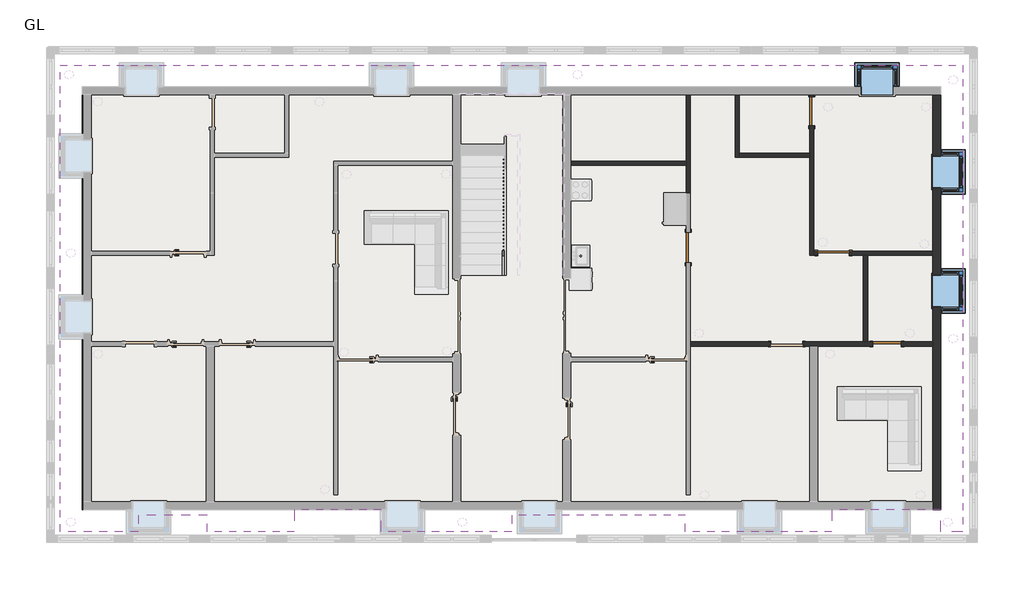
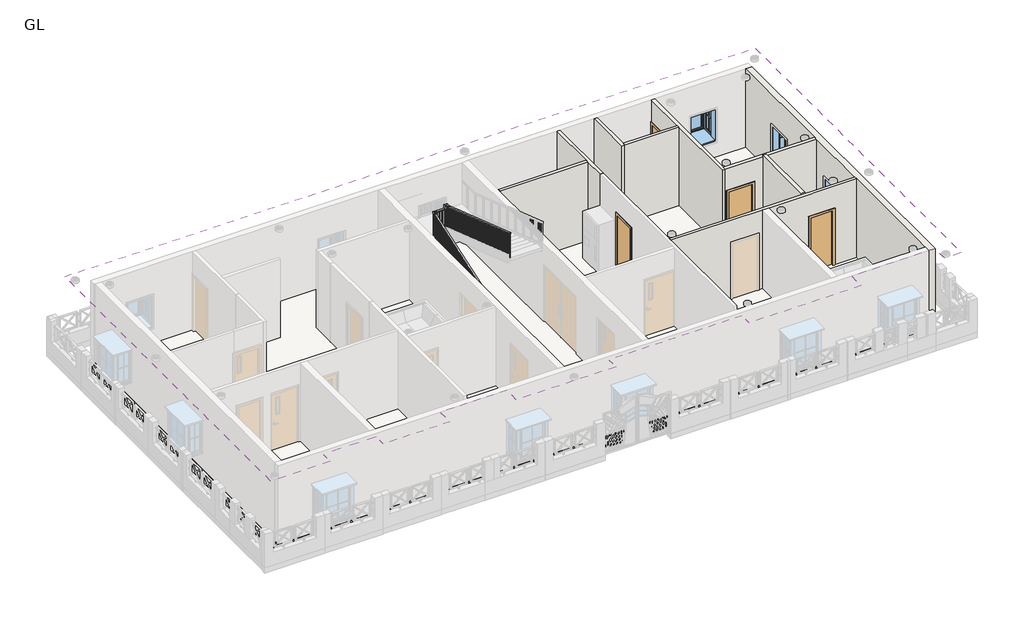
# One storey, part 2 of 5: 10 walls, 4 doors, 3 windows, 1 covering, 1 railing, 1 slab.
"""IFC4 building model written with IfcOpenShell, lengths in millimetres."""

from ifc_helpers import new_model, si_unit, frame, origin, origin_with_axes, place, context, project, spatial, polyline, outline, extrude, faceted_brep, transform, mapped, element, save
from components import door_700d3439, door_8cb1b8a7, door_38851409, door_d141acb4, window_bay_casement_box_90_degree_angle_center_fixed_4_x3_2dea7aab

model = new_model("IFC4")

# Units and contexts
model_context = context("Model", 3, world=origin())
ifc_project = project(units=[si_unit("LENGTHUNIT", "METRE", prefix="MILLI")], contexts=[model_context])

# Site, building, storey
site = spatial("IfcSite", under=ifc_project)
building = spatial("IfcBuilding", under=site)
storey = spatial("IfcBuildingStorey", under=building, Name="GL", Elevation=0.0)

# Covering
placement = place(None, origin())
element("IfcCovering", 1, ObjectType="2' x 4' ACT System", at=placement, inside=storey, context=model_context, shape_type="SweptSolid", body=[
    extrude(outline(polyline([(12235.5012075, 8470.0067329), (12235.5012075, -4623.6932193), (11625.9012075, -4623.6932193), (11625.9012075, -4014.0932193), (8564.9472043, -4014.0932193), (8564.9472043, -4623.6932193), (4450.1472043, -4623.6932193), (4450.1472043, -4172.8432432), (-426.6527957, -4172.8432432), (-426.6527957, -4623.6932193), (-4084.2527957, -4623.6932193), (-4084.2527957, -4014.0932193), (-6522.6527957, -4014.0932193), (-6522.6527957, -4623.6932193), (-8961.0527957, -4623.6932193), (-8961.0527957, -4172.8432432), (-10904.4067989, -4172.8432432), (-10904.4067989, -4623.6932193), (-13088.8067989, -4623.6932193), (-13088.8067989, 8470.0067329), (12235.5012075, 8470.0067329)])), frame((0.0, 0.0, 3048.0), z_axis=(0.0, 0.0, 1.0), x_axis=(1.0, 0.0, 0.0)), (0.0, 0.0, 1.0), 57.15),
])

# Doors
door_shape = door_700d3439(model_context)
element("IfcDoor", 2, ObjectType="Single-Flush : 2'10\" x 7'", at=placement, inside=storey, context=model_context, shape_type="MappedRepresentation", body=[
    mapped(door_shape, transform((4532.9512082, 3351.906733, 0.0), x_axis=(0.0, -1.0, 0.0), y_axis=(1.0, 0.0, 0.0), z_axis=(0.0, 0.0, 1.0))),
])
door_2_shape = door_8cb1b8a7(model_context)
element("IfcDoor", 3, ObjectType="Single-Flush : 2'11\"x 7'", at=placement, inside=storey, context=model_context, shape_type="MappedRepresentation", body=[
    mapped(door_2_shape, transform((8609.6512079, 3193.1567332, 0.0), x_axis=(-1.0, 0.0, 0.0), y_axis=(0.0, -1.0, 0.0), z_axis=(0.0, 0.0, 1.0))),
])
door_3_shape = door_38851409(model_context)
element("IfcDoor", 4, ObjectType="Single-Flush : 2'8\"x 7'", at=placement, inside=storey, context=model_context, shape_type="MappedRepresentation", body=[
    mapped(door_3_shape, transform((10111.5098918, 640.4567334, 0.0), x_axis=(-1.0, 0.0, 0.0), y_axis=(0.0, -1.0, 0.0), z_axis=(0.0, 0.0, 1.0))),
])
door_4_shape = door_d141acb4(model_context)
element("IfcDoor", 5, ObjectType="Single-Flush : 2'8\"x 7'", at=placement, inside=storey, context=model_context, shape_type="MappedRepresentation", body=[
    mapped(door_4_shape, transform((8000.0512079, 7167.840939, 0.0), x_axis=(0.0, 1.0, 0.0), y_axis=(-1.0, 0.0, 0.0), z_axis=(0.0, 0.0, 1.0))),
])

# Railing
element("IfcRailing", 6, ObjectType="Handrail - Rectangular", at=placement, inside=storey, context=model_context, shape_type="SolidModel", body=[
    faceted_brep([(-680.3987998, 2564.5067329, 1017.8142857), (-680.3987998, 2564.5067329, 964.1699957), (-629.5987998, 2564.5067329, 964.1699957), (-629.5987998, 2564.5067329, 1017.8142857), (-680.3987998, 6450.7067329, 2336.3464286), (-680.3987998, 6501.5067329, 2299.9378529), (-629.5987998, 6501.5067329, 2299.9378529), (-629.5987998, 6450.7067329, 2336.3464286), (-553.3987998, 6577.7067329, 2311.4), (-553.3987998, 6577.7067329, 2362.2), (-273.9987915, 6577.7067329, 2362.2), (-223.1987915, 6577.7067329, 2311.4), (-553.3987998, 6526.9067329, 2311.4), (-223.1987915, 6526.9067329, 2311.4), (-553.3987998, 6526.9067329, 2362.2), (-273.9987915, 6526.9067329, 2362.2), (-146.9987915, 2564.5067329, 3810.0), (-197.7987915, 2564.5067329, 3810.0), (-197.7987915, 2564.5067329, 3756.35571), (-146.9987915, 2564.5067329, 3756.35571), (-146.9987915, 6442.3235624, 2440.6678571), (-146.9987915, 6450.7067329, 2491.4678571), (-197.7987915, 6442.3235624, 2440.6678571), (-197.7987915, 6450.7067329, 2491.4678571), (-680.3987998, 6450.7067329, 2362.2), (-680.3987998, 6501.5067329, 2311.4), (-629.5987998, 6501.5067329, 2311.4), (-629.5987998, 6450.7067329, 2362.2), (-680.3987998, 6577.7067329, 2362.2), (-680.3987998, 6577.7067329, 2311.4), (-629.5987998, 6526.9067329, 2311.4), (-629.5987998, 6526.9067329, 2362.2), (-273.9987915, 6577.7067329, 2491.4678571), (-223.1987915, 6577.7067329, 2440.6678571), (-223.1987915, 6526.9067329, 2440.6678571), (-273.9987915, 6526.9067329, 2491.4678571), (-146.9987915, 6577.7067329, 2491.4678571), (-146.9987915, 6577.7067329, 2440.6678571), (-197.7987915, 6526.9067329, 2440.6678571), (-197.7987915, 6526.9067329, 2491.4678571)], [[[0, 1, 2, 3]], [[1, 0, 4, 5]], [[2, 1, 5, 6]], [[3, 2, 6, 7]], [[0, 3, 7, 4]], [[8, 9, 10, 11]], [[12, 8, 11, 13]], [[14, 12, 13, 15]], [[9, 14, 15, 10]], [[16, 17, 18, 19]], [[20, 21, 16, 19]], [[22, 20, 19, 18]], [[23, 22, 18, 17]], [[21, 23, 17, 16]], [[5, 4, 24, 25]], [[6, 5, 25, 26]], [[7, 6, 26, 27]], [[4, 7, 27, 24]], [[25, 24, 28, 29]], [[26, 25, 29, 30]], [[27, 26, 30, 31]], [[24, 27, 31, 28]], [[29, 28, 9, 8]], [[30, 29, 8, 12]], [[31, 30, 12, 14]], [[28, 31, 14, 9]], [[11, 10, 32, 33]], [[13, 11, 33, 34]], [[15, 13, 34, 35]], [[10, 15, 35, 32]], [[33, 32, 36, 37]], [[34, 33, 37, 38]], [[35, 34, 38, 39]], [[32, 35, 39, 36]], [[37, 36, 21, 20]], [[38, 37, 20, 22]], [[39, 38, 22, 23]], [[36, 39, 23, 21]]]),
    extrude(outline(polyline([(2580.3817329, 3750.9695493), (2599.4317329, 3744.5061565), (2599.4317329, 2792.1857143), (2580.3817329, 2792.1857143), (2580.3817329, 3750.9695493)])), frame((-181.9237915, 0.0, 0.0), z_axis=(1.0, 0.0, 0.0), x_axis=(0.0, 1.0, 0.0)), (0.0, 0.0, 1.0), 19.05),
    extrude(outline(polyline([(2681.9817329, 3716.4981207), (2701.0317329, 3710.0347279), (2701.0317329, 2792.1857143), (2681.9817329, 2792.1857143), (2681.9817329, 3716.4981207)])), frame((-181.9237915, 0.0, 0.0), z_axis=(1.0, 0.0, 0.0), x_axis=(0.0, 1.0, 0.0)), (0.0, 0.0, 1.0), 19.05),
    extrude(outline(polyline([(2783.5817329, 3682.0266922), (2802.6317329, 3675.5632993), (2802.6317329, 2792.1857143), (2783.5817329, 2792.1857143), (2783.5817329, 3682.0266922)])), frame((-181.9237915, 0.0, 0.0), z_axis=(1.0, 0.0, 0.0), x_axis=(0.0, 1.0, 0.0)), (0.0, 0.0, 1.0), 19.05),
    extrude(outline(polyline([(2885.1817329, 3647.5552636), (2904.2317329, 3641.0918707), (2904.2317329, 2688.7714286), (2885.1817329, 2688.7714286), (2885.1817329, 3647.5552636)])), frame((-181.9237915, 0.0, 0.0), z_axis=(1.0, 0.0, 0.0), x_axis=(0.0, 1.0, 0.0)), (0.0, 0.0, 1.0), 19.05),
    extrude(outline(polyline([(2986.7817329, 3613.083835), (3005.8317329, 3606.6204422), (3005.8317329, 2688.7714286), (2986.7817329, 2688.7714286), (2986.7817329, 3613.083835)])), frame((-181.9237915, 0.0, 0.0), z_axis=(1.0, 0.0, 0.0), x_axis=(0.0, 1.0, 0.0)), (0.0, 0.0, 1.0), 19.05),
    extrude(outline(polyline([(3088.3817329, 3578.6124065), (3107.4317329, 3572.1490136), (3107.4317329, 2688.7714286), (3088.3817329, 2688.7714286), (3088.3817329, 3578.6124065)])), frame((-181.9237915, 0.0, 0.0), z_axis=(1.0, 0.0, 0.0), x_axis=(0.0, 1.0, 0.0)), (0.0, 0.0, 1.0), 19.05),
    extrude(outline(polyline([(3189.9817329, 3544.1409779), (3209.0317329, 3537.677585), (3209.0317329, 2585.3571429), (3189.9817329, 2585.3571429), (3189.9817329, 3544.1409779)])), frame((-181.9237915, 0.0, 0.0), z_axis=(1.0, 0.0, 0.0), x_axis=(0.0, 1.0, 0.0)), (0.0, 0.0, 1.0), 19.05),
    extrude(outline(polyline([(3291.5817329, 3509.6695493), (3310.6317329, 3503.2061565), (3310.6317329, 2585.3571429), (3291.5817329, 2585.3571429), (3291.5817329, 3509.6695493)])), frame((-181.9237915, 0.0, 0.0), z_axis=(1.0, 0.0, 0.0), x_axis=(0.0, 1.0, 0.0)), (0.0, 0.0, 1.0), 19.05),
    extrude(outline(polyline([(3393.1817329, 3475.1981207), (3412.2317329, 3468.7347279), (3412.2317329, 2585.3571429), (3393.1817329, 2585.3571429), (3393.1817329, 3475.1981207)])), frame((-181.9237915, 0.0, 0.0), z_axis=(1.0, 0.0, 0.0), x_axis=(0.0, 1.0, 0.0)), (0.0, 0.0, 1.0), 19.05),
    extrude(outline(polyline([(3494.7817329, 3440.7266922), (3513.8317329, 3434.2632993), (3513.8317329, 2481.9428571), (3494.7817329, 2481.9428571), (3494.7817329, 3440.7266922)])), frame((-181.9237915, 0.0, 0.0), z_axis=(1.0, 0.0, 0.0), x_axis=(0.0, 1.0, 0.0)), (0.0, 0.0, 1.0), 19.05),
    extrude(outline(polyline([(3596.3817329, 3406.2552636), (3615.4317329, 3399.7918707), (3615.4317329, 2481.9428571), (3596.3817329, 2481.9428571), (3596.3817329, 3406.2552636)])), frame((-181.9237915, 0.0, 0.0), z_axis=(1.0, 0.0, 0.0), x_axis=(0.0, 1.0, 0.0)), (0.0, 0.0, 1.0), 19.05),
    extrude(outline(polyline([(3697.9817329, 3371.783835), (3717.0317329, 3365.3204422), (3717.0317329, 2481.9428571), (3697.9817329, 2481.9428571), (3697.9817329, 3371.783835)])), frame((-181.9237915, 0.0, 0.0), z_axis=(1.0, 0.0, 0.0), x_axis=(0.0, 1.0, 0.0)), (0.0, 0.0, 1.0), 19.05),
    extrude(outline(polyline([(3799.5817329, 3337.3124065), (3818.6317329, 3330.8490136), (3818.6317329, 2378.5285714), (3799.5817329, 2378.5285714), (3799.5817329, 3337.3124065)])), frame((-181.9237915, 0.0, 0.0), z_axis=(1.0, 0.0, 0.0), x_axis=(0.0, 1.0, 0.0)), (0.0, 0.0, 1.0), 19.05),
    extrude(outline(polyline([(3901.1817329, 3302.8409779), (3920.2317329, 3296.377585), (3920.2317329, 2378.5285714), (3901.1817329, 2378.5285714), (3901.1817329, 3302.8409779)])), frame((-181.9237915, 0.0, 0.0), z_axis=(1.0, 0.0, 0.0), x_axis=(0.0, 1.0, 0.0)), (0.0, 0.0, 1.0), 19.05),
    extrude(outline(polyline([(4002.7817329, 3268.3695493), (4021.8317329, 3261.9061565), (4021.8317329, 2378.5285714), (4002.7817329, 2378.5285714), (4002.7817329, 3268.3695493)])), frame((-181.9237915, 0.0, 0.0), z_axis=(1.0, 0.0, 0.0), x_axis=(0.0, 1.0, 0.0)), (0.0, 0.0, 1.0), 19.05),
    extrude(outline(polyline([(4104.3817329, 3233.8981207), (4123.4317329, 3227.4347279), (4123.4317329, 2275.1142857), (4104.3817329, 2275.1142857), (4104.3817329, 3233.8981207)])), frame((-181.9237915, 0.0, 0.0), z_axis=(1.0, 0.0, 0.0), x_axis=(0.0, 1.0, 0.0)), (0.0, 0.0, 1.0), 19.05),
    extrude(outline(polyline([(4205.9817329, 3199.4266922), (4225.0317329, 3192.9632993), (4225.0317329, 2275.1142857), (4205.9817329, 2275.1142857), (4205.9817329, 3199.4266922)])), frame((-181.9237915, 0.0, 0.0), z_axis=(1.0, 0.0, 0.0), x_axis=(0.0, 1.0, 0.0)), (0.0, 0.0, 1.0), 19.05),
    extrude(outline(polyline([(4307.5817329, 3164.9552636), (4326.6317329, 3158.4918707), (4326.6317329, 2275.1142857), (4307.5817329, 2275.1142857), (4307.5817329, 3164.9552636)])), frame((-181.9237915, 0.0, 0.0), z_axis=(1.0, 0.0, 0.0), x_axis=(0.0, 1.0, 0.0)), (0.0, 0.0, 1.0), 19.05),
    extrude(outline(polyline([(4409.1817329, 3130.483835), (4428.2317329, 3124.0204422), (4428.2317329, 2171.7), (4409.1817329, 2171.7), (4409.1817329, 3130.483835)])), frame((-181.9237915, 0.0, 0.0), z_axis=(1.0, 0.0, 0.0), x_axis=(0.0, 1.0, 0.0)), (0.0, 0.0, 1.0), 19.05),
    extrude(outline(polyline([(4510.7817329, 3096.0124065), (4529.8317329, 3089.5490136), (4529.8317329, 2171.7), (4510.7817329, 2171.7), (4510.7817329, 3096.0124065)])), frame((-181.9237915, 0.0, 0.0), z_axis=(1.0, 0.0, 0.0), x_axis=(0.0, 1.0, 0.0)), (0.0, 0.0, 1.0), 19.05),
    extrude(outline(polyline([(4612.3817329, 3061.5409779), (4631.4317329, 3055.077585), (4631.4317329, 2171.7), (4612.3817329, 2171.7), (4612.3817329, 3061.5409779)])), frame((-181.9237915, 0.0, 0.0), z_axis=(1.0, 0.0, 0.0), x_axis=(0.0, 1.0, 0.0)), (0.0, 0.0, 1.0), 19.05),
    extrude(outline(polyline([(4713.9817329, 3027.0695493), (4733.0317329, 3020.6061565), (4733.0317329, 2068.2857143), (4713.9817329, 2068.2857143), (4713.9817329, 3027.0695493)])), frame((-181.9237915, 0.0, 0.0), z_axis=(1.0, 0.0, 0.0), x_axis=(0.0, 1.0, 0.0)), (0.0, 0.0, 1.0), 19.05),
    extrude(outline(polyline([(4815.5817329, 2992.5981207), (4834.6317329, 2986.1347279), (4834.6317329, 2068.2857143), (4815.5817329, 2068.2857143), (4815.5817329, 2992.5981207)])), frame((-181.9237915, 0.0, 0.0), z_axis=(1.0, 0.0, 0.0), x_axis=(0.0, 1.0, 0.0)), (0.0, 0.0, 1.0), 19.05),
    extrude(outline(polyline([(4917.1817329, 2958.1266922), (4936.2317329, 2951.6632993), (4936.2317329, 2068.2857143), (4917.1817329, 2068.2857143), (4917.1817329, 2958.1266922)])), frame((-181.9237915, 0.0, 0.0), z_axis=(1.0, 0.0, 0.0), x_axis=(0.0, 1.0, 0.0)), (0.0, 0.0, 1.0), 19.05),
    extrude(outline(polyline([(5018.7817329, 2923.6552636), (5037.8317329, 2917.1918707), (5037.8317329, 1964.8714286), (5018.7817329, 1964.8714286), (5018.7817329, 2923.6552636)])), frame((-181.9237915, 0.0, 0.0), z_axis=(1.0, 0.0, 0.0), x_axis=(0.0, 1.0, 0.0)), (0.0, 0.0, 1.0), 19.05),
    extrude(outline(polyline([(5120.3817329, 2889.183835), (5139.4317329, 2882.7204422), (5139.4317329, 1964.8714286), (5120.3817329, 1964.8714286), (5120.3817329, 2889.183835)])), frame((-181.9237915, 0.0, 0.0), z_axis=(1.0, 0.0, 0.0), x_axis=(0.0, 1.0, 0.0)), (0.0, 0.0, 1.0), 19.05),
    extrude(outline(polyline([(5221.9817329, 2854.7124065), (5241.0317329, 2848.2490136), (5241.0317329, 1964.8714286), (5221.9817329, 1964.8714286), (5221.9817329, 2854.7124065)])), frame((-181.9237915, 0.0, 0.0), z_axis=(1.0, 0.0, 0.0), x_axis=(0.0, 1.0, 0.0)), (0.0, 0.0, 1.0), 19.05),
    extrude(outline(polyline([(5323.5817329, 2820.2409779), (5342.6317329, 2813.777585), (5342.6317329, 1861.4571429), (5323.5817329, 1861.4571429), (5323.5817329, 2820.2409779)])), frame((-181.9237915, 0.0, 0.0), z_axis=(1.0, 0.0, 0.0), x_axis=(0.0, 1.0, 0.0)), (0.0, 0.0, 1.0), 19.05),
    extrude(outline(polyline([(5425.1817329, 2785.7695493), (5444.2317329, 2779.3061565), (5444.2317329, 1861.4571429), (5425.1817329, 1861.4571429), (5425.1817329, 2785.7695493)])), frame((-181.9237915, 0.0, 0.0), z_axis=(1.0, 0.0, 0.0), x_axis=(0.0, 1.0, 0.0)), (0.0, 0.0, 1.0), 19.05),
    extrude(outline(polyline([(5526.7817329, 2751.2981207), (5545.8317329, 2744.8347279), (5545.8317329, 1861.4571429), (5526.7817329, 1861.4571429), (5526.7817329, 2751.2981207)])), frame((-181.9237915, 0.0, 0.0), z_axis=(1.0, 0.0, 0.0), x_axis=(0.0, 1.0, 0.0)), (0.0, 0.0, 1.0), 19.05),
    extrude(outline(polyline([(5628.3817329, 2716.8266922), (5647.4317329, 2710.3632993), (5647.4317329, 1758.0428571), (5628.3817329, 1758.0428571), (5628.3817329, 2716.8266922)])), frame((-181.9237915, 0.0, 0.0), z_axis=(1.0, 0.0, 0.0), x_axis=(0.0, 1.0, 0.0)), (0.0, 0.0, 1.0), 19.05),
    extrude(outline(polyline([(5729.9817329, 2682.3552636), (5749.0317329, 2675.8918707), (5749.0317329, 1758.0428571), (5729.9817329, 1758.0428571), (5729.9817329, 2682.3552636)])), frame((-181.9237915, 0.0, 0.0), z_axis=(1.0, 0.0, 0.0), x_axis=(0.0, 1.0, 0.0)), (0.0, 0.0, 1.0), 19.05),
    extrude(outline(polyline([(5831.5817329, 2647.883835), (5850.6317329, 2641.4204422), (5850.6317329, 1758.0428571), (5831.5817329, 1758.0428571), (5831.5817329, 2647.883835)])), frame((-181.9237915, 0.0, 0.0), z_axis=(1.0, 0.0, 0.0), x_axis=(0.0, 1.0, 0.0)), (0.0, 0.0, 1.0), 19.05),
    extrude(outline(polyline([(5933.1817329, 2613.4124065), (5952.2317329, 2606.9490136), (5952.2317329, 1654.6285714), (5933.1817329, 1654.6285714), (5933.1817329, 2613.4124065)])), frame((-181.9237915, 0.0, 0.0), z_axis=(1.0, 0.0, 0.0), x_axis=(0.0, 1.0, 0.0)), (0.0, 0.0, 1.0), 19.05),
    extrude(outline(polyline([(6034.7817329, 2578.9409779), (6053.8317329, 2572.477585), (6053.8317329, 1654.6285714), (6034.7817329, 1654.6285714), (6034.7817329, 2578.9409779)])), frame((-181.9237915, 0.0, 0.0), z_axis=(1.0, 0.0, 0.0), x_axis=(0.0, 1.0, 0.0)), (0.0, 0.0, 1.0), 19.05),
    extrude(outline(polyline([(6136.3817329, 2544.4695493), (6155.4317329, 2538.0061565), (6155.4317329, 1654.6285714), (6136.3817329, 1654.6285714), (6136.3817329, 2544.4695493)])), frame((-181.9237915, 0.0, 0.0), z_axis=(1.0, 0.0, 0.0), x_axis=(0.0, 1.0, 0.0)), (0.0, 0.0, 1.0), 19.05),
    extrude(outline(polyline([(6237.9817329, 2509.9981207), (6257.0317329, 2503.5347279), (6257.0317329, 1551.2142857), (6237.9817329, 1551.2142857), (6237.9817329, 2509.9981207)])), frame((-181.9237915, 0.0, 0.0), z_axis=(1.0, 0.0, 0.0), x_axis=(0.0, 1.0, 0.0)), (0.0, 0.0, 1.0), 19.05),
    extrude(outline(polyline([(6339.5817329, 2475.5266922), (6358.6317329, 2469.0632993), (6358.6317329, 1551.2142857), (6339.5817329, 1551.2142857), (6339.5817329, 2475.5266922)])), frame((-181.9237915, 0.0, 0.0), z_axis=(1.0, 0.0, 0.0), x_axis=(0.0, 1.0, 0.0)), (0.0, 0.0, 1.0), 19.05),
    extrude(outline(polyline([(6441.1817329, 2441.0552636), (6460.2317329, 2434.5918707), (6460.2317329, 1551.2142857), (6441.1817329, 1551.2142857), (6441.1817329, 2441.0552636)])), frame((-181.9237915, 0.0, 0.0), z_axis=(1.0, 0.0, 0.0), x_axis=(0.0, 1.0, 0.0)), (0.0, 0.0, 1.0), 19.05),
    extrude(outline(polyline([(-258.1237998, 6542.7817329), (-258.1237998, 6561.8317329), (-239.0737998, 6561.8317329), (-239.0737998, 6542.7817329), (-258.1237998, 6542.7817329)])), frame((0.0, 0.0, 1447.8), z_axis=(0.0, 0.0, 1.0), x_axis=(1.0, 0.0, 0.0)), (0.0, 0.0, 1.0), 992.8678571),
    extrude(outline(polyline([(-359.7237998, 6542.7817329), (-359.7237998, 6561.8317329), (-340.6737998, 6561.8317329), (-340.6737998, 6542.7817329), (-359.7237998, 6542.7817329)])), frame((0.0, 0.0, 1447.8), z_axis=(0.0, 0.0, 1.0), x_axis=(1.0, 0.0, 0.0)), (0.0, 0.0, 1.0), 863.6),
    extrude(outline(polyline([(-461.3237998, 6542.7817329), (-461.3237998, 6561.8317329), (-442.2737998, 6561.8317329), (-442.2737998, 6542.7817329), (-461.3237998, 6542.7817329)])), frame((0.0, 0.0, 1447.8), z_axis=(0.0, 0.0, 1.0), x_axis=(1.0, 0.0, 0.0)), (0.0, 0.0, 1.0), 863.6),
    extrude(outline(polyline([(-562.9237998, 6542.7817329), (-562.9237998, 6561.8317329), (-543.8737998, 6561.8317329), (-543.8737998, 6542.7817329), (-562.9237998, 6542.7817329)])), frame((0.0, 0.0, 1447.8), z_axis=(0.0, 0.0, 1.0), x_axis=(1.0, 0.0, 0.0)), (0.0, 0.0, 1.0), 863.6),
    extrude(outline(polyline([(-645.4737998, 6517.3817329), (-664.5237998, 6517.3817329), (-664.5237998, 6536.4317329), (-645.4737998, 6536.4317329), (-645.4737998, 6517.3817329)])), frame((0.0, 0.0, 1447.8), z_axis=(0.0, 0.0, 1.0), x_axis=(1.0, 0.0, 0.0)), (0.0, 0.0, 1.0), 863.6),
    extrude(outline(polyline([(6415.7817329, 2270.852585), (6434.8317329, 2277.3159779), (6434.8317329, 1344.3857143), (6415.7817329, 1344.3857143), (6415.7817329, 2270.852585)])), frame((-664.5237998, 0.0, 0.0), z_axis=(1.0, 0.0, 0.0), x_axis=(0.0, 1.0, 0.0)), (0.0, 0.0, 1.0), 19.05),
    extrude(outline(polyline([(6314.1817329, 2236.3811565), (6333.2317329, 2242.8445493), (6333.2317329, 1344.3857143), (6314.1817329, 1344.3857143), (6314.1817329, 2236.3811565)])), frame((-664.5237998, 0.0, 0.0), z_axis=(1.0, 0.0, 0.0), x_axis=(0.0, 1.0, 0.0)), (0.0, 0.0, 1.0), 19.05),
    extrude(outline(polyline([(6212.5817329, 2201.9097279), (6231.6317329, 2208.3731207), (6231.6317329, 1344.3857143), (6212.5817329, 1344.3857143), (6212.5817329, 2201.9097279)])), frame((-664.5237998, 0.0, 0.0), z_axis=(1.0, 0.0, 0.0), x_axis=(0.0, 1.0, 0.0)), (0.0, 0.0, 1.0), 19.05),
    extrude(outline(polyline([(6110.9817329, 2167.4382993), (6130.0317329, 2173.9016922), (6130.0317329, 1240.9714286), (6110.9817329, 1240.9714286), (6110.9817329, 2167.4382993)])), frame((-664.5237998, 0.0, 0.0), z_axis=(1.0, 0.0, 0.0), x_axis=(0.0, 1.0, 0.0)), (0.0, 0.0, 1.0), 19.05),
    extrude(outline(polyline([(6009.3817329, 2132.9668707), (6028.4317329, 2139.4302636), (6028.4317329, 1240.9714286), (6009.3817329, 1240.9714286), (6009.3817329, 2132.9668707)])), frame((-664.5237998, 0.0, 0.0), z_axis=(1.0, 0.0, 0.0), x_axis=(0.0, 1.0, 0.0)), (0.0, 0.0, 1.0), 19.05),
    extrude(outline(polyline([(5907.7817329, 2098.4954422), (5926.8317329, 2104.958835), (5926.8317329, 1240.9714286), (5907.7817329, 1240.9714286), (5907.7817329, 2098.4954422)])), frame((-664.5237998, 0.0, 0.0), z_axis=(1.0, 0.0, 0.0), x_axis=(0.0, 1.0, 0.0)), (0.0, 0.0, 1.0), 19.05),
    extrude(outline(polyline([(5806.1817329, 2064.0240136), (5825.2317329, 2070.4874065), (5825.2317329, 1137.5571429), (5806.1817329, 1137.5571429), (5806.1817329, 2064.0240136)])), frame((-664.5237998, 0.0, 0.0), z_axis=(1.0, 0.0, 0.0), x_axis=(0.0, 1.0, 0.0)), (0.0, 0.0, 1.0), 19.05),
    extrude(outline(polyline([(5704.5817329, 2029.552585), (5723.6317329, 2036.0159779), (5723.6317329, 1137.5571429), (5704.5817329, 1137.5571429), (5704.5817329, 2029.552585)])), frame((-664.5237998, 0.0, 0.0), z_axis=(1.0, 0.0, 0.0), x_axis=(0.0, 1.0, 0.0)), (0.0, 0.0, 1.0), 19.05),
    extrude(outline(polyline([(5602.9817329, 1995.0811565), (5622.0317329, 2001.5445493), (5622.0317329, 1137.5571429), (5602.9817329, 1137.5571429), (5602.9817329, 1995.0811565)])), frame((-664.5237998, 0.0, 0.0), z_axis=(1.0, 0.0, 0.0), x_axis=(0.0, 1.0, 0.0)), (0.0, 0.0, 1.0), 19.05),
    extrude(outline(polyline([(5501.3817329, 1960.6097279), (5520.4317329, 1967.0731207), (5520.4317329, 1034.1428571), (5501.3817329, 1034.1428571), (5501.3817329, 1960.6097279)])), frame((-664.5237998, 0.0, 0.0), z_axis=(1.0, 0.0, 0.0), x_axis=(0.0, 1.0, 0.0)), (0.0, 0.0, 1.0), 19.05),
    extrude(outline(polyline([(5399.7817329, 1926.1382993), (5418.8317329, 1932.6016922), (5418.8317329, 1034.1428571), (5399.7817329, 1034.1428571), (5399.7817329, 1926.1382993)])), frame((-664.5237998, 0.0, 0.0), z_axis=(1.0, 0.0, 0.0), x_axis=(0.0, 1.0, 0.0)), (0.0, 0.0, 1.0), 19.05),
    extrude(outline(polyline([(5298.1817329, 1891.6668707), (5317.2317329, 1898.1302636), (5317.2317329, 1034.1428571), (5298.1817329, 1034.1428571), (5298.1817329, 1891.6668707)])), frame((-664.5237998, 0.0, 0.0), z_axis=(1.0, 0.0, 0.0), x_axis=(0.0, 1.0, 0.0)), (0.0, 0.0, 1.0), 19.05),
    extrude(outline(polyline([(5196.5817329, 1857.1954422), (5215.6317329, 1863.658835), (5215.6317329, 930.7285714), (5196.5817329, 930.7285714), (5196.5817329, 1857.1954422)])), frame((-664.5237998, 0.0, 0.0), z_axis=(1.0, 0.0, 0.0), x_axis=(0.0, 1.0, 0.0)), (0.0, 0.0, 1.0), 19.05),
    extrude(outline(polyline([(5094.9817329, 1822.7240136), (5114.0317329, 1829.1874065), (5114.0317329, 930.7285714), (5094.9817329, 930.7285714), (5094.9817329, 1822.7240136)])), frame((-664.5237998, 0.0, 0.0), z_axis=(1.0, 0.0, 0.0), x_axis=(0.0, 1.0, 0.0)), (0.0, 0.0, 1.0), 19.05),
    extrude(outline(polyline([(4993.3817329, 1788.252585), (5012.4317329, 1794.7159779), (5012.4317329, 930.7285714), (4993.3817329, 930.7285714), (4993.3817329, 1788.252585)])), frame((-664.5237998, 0.0, 0.0), z_axis=(1.0, 0.0, 0.0), x_axis=(0.0, 1.0, 0.0)), (0.0, 0.0, 1.0), 19.05),
    extrude(outline(polyline([(4891.7817329, 1753.7811565), (4910.8317329, 1760.2445493), (4910.8317329, 827.3142857), (4891.7817329, 827.3142857), (4891.7817329, 1753.7811565)])), frame((-664.5237998, 0.0, 0.0), z_axis=(1.0, 0.0, 0.0), x_axis=(0.0, 1.0, 0.0)), (0.0, 0.0, 1.0), 19.05),
    extrude(outline(polyline([(4790.1817329, 1719.3097279), (4809.2317329, 1725.7731207), (4809.2317329, 827.3142857), (4790.1817329, 827.3142857), (4790.1817329, 1719.3097279)])), frame((-664.5237998, 0.0, 0.0), z_axis=(1.0, 0.0, 0.0), x_axis=(0.0, 1.0, 0.0)), (0.0, 0.0, 1.0), 19.05),
    extrude(outline(polyline([(4688.5817329, 1684.8382993), (4707.6317329, 1691.3016922), (4707.6317329, 827.3142857), (4688.5817329, 827.3142857), (4688.5817329, 1684.8382993)])), frame((-664.5237998, 0.0, 0.0), z_axis=(1.0, 0.0, 0.0), x_axis=(0.0, 1.0, 0.0)), (0.0, 0.0, 1.0), 19.05),
    extrude(outline(polyline([(4586.9817329, 1650.3668707), (4606.0317329, 1656.8302636), (4606.0317329, 723.9), (4586.9817329, 723.9), (4586.9817329, 1650.3668707)])), frame((-664.5237998, 0.0, 0.0), z_axis=(1.0, 0.0, 0.0), x_axis=(0.0, 1.0, 0.0)), (0.0, 0.0, 1.0), 19.05),
    extrude(outline(polyline([(4485.3817329, 1615.8954422), (4504.4317329, 1622.358835), (4504.4317329, 723.9), (4485.3817329, 723.9), (4485.3817329, 1615.8954422)])), frame((-664.5237998, 0.0, 0.0), z_axis=(1.0, 0.0, 0.0), x_axis=(0.0, 1.0, 0.0)), (0.0, 0.0, 1.0), 19.05),
    extrude(outline(polyline([(4383.7817329, 1581.4240136), (4402.8317329, 1587.8874065), (4402.8317329, 723.9), (4383.7817329, 723.9), (4383.7817329, 1581.4240136)])), frame((-664.5237998, 0.0, 0.0), z_axis=(1.0, 0.0, 0.0), x_axis=(0.0, 1.0, 0.0)), (0.0, 0.0, 1.0), 19.05),
    extrude(outline(polyline([(4282.1817329, 1546.952585), (4301.2317329, 1553.4159779), (4301.2317329, 620.4857143), (4282.1817329, 620.4857143), (4282.1817329, 1546.952585)])), frame((-664.5237998, 0.0, 0.0), z_axis=(1.0, 0.0, 0.0), x_axis=(0.0, 1.0, 0.0)), (0.0, 0.0, 1.0), 19.05),
    extrude(outline(polyline([(4180.5817329, 1512.4811565), (4199.6317329, 1518.9445493), (4199.6317329, 620.4857143), (4180.5817329, 620.4857143), (4180.5817329, 1512.4811565)])), frame((-664.5237998, 0.0, 0.0), z_axis=(1.0, 0.0, 0.0), x_axis=(0.0, 1.0, 0.0)), (0.0, 0.0, 1.0), 19.05),
    extrude(outline(polyline([(4078.9817329, 1478.0097279), (4098.0317329, 1484.4731207), (4098.0317329, 620.4857143), (4078.9817329, 620.4857143), (4078.9817329, 1478.0097279)])), frame((-664.5237998, 0.0, 0.0), z_axis=(1.0, 0.0, 0.0), x_axis=(0.0, 1.0, 0.0)), (0.0, 0.0, 1.0), 19.05),
    extrude(outline(polyline([(3977.3817329, 1443.5382993), (3996.4317329, 1450.0016922), (3996.4317329, 517.0714286), (3977.3817329, 517.0714286), (3977.3817329, 1443.5382993)])), frame((-664.5237998, 0.0, 0.0), z_axis=(1.0, 0.0, 0.0), x_axis=(0.0, 1.0, 0.0)), (0.0, 0.0, 1.0), 19.05),
    extrude(outline(polyline([(3875.7817329, 1409.0668707), (3894.8317329, 1415.5302636), (3894.8317329, 517.0714286), (3875.7817329, 517.0714286), (3875.7817329, 1409.0668707)])), frame((-664.5237998, 0.0, 0.0), z_axis=(1.0, 0.0, 0.0), x_axis=(0.0, 1.0, 0.0)), (0.0, 0.0, 1.0), 19.05),
    extrude(outline(polyline([(3774.1817329, 1374.5954422), (3793.2317329, 1381.058835), (3793.2317329, 517.0714286), (3774.1817329, 517.0714286), (3774.1817329, 1374.5954422)])), frame((-664.5237998, 0.0, 0.0), z_axis=(1.0, 0.0, 0.0), x_axis=(0.0, 1.0, 0.0)), (0.0, 0.0, 1.0), 19.05),
    extrude(outline(polyline([(3672.5817329, 1340.1240136), (3691.6317329, 1346.5874065), (3691.6317329, 413.6571429), (3672.5817329, 413.6571429), (3672.5817329, 1340.1240136)])), frame((-664.5237998, 0.0, 0.0), z_axis=(1.0, 0.0, 0.0), x_axis=(0.0, 1.0, 0.0)), (0.0, 0.0, 1.0), 19.05),
    extrude(outline(polyline([(3570.9817329, 1305.652585), (3590.0317329, 1312.1159779), (3590.0317329, 413.6571429), (3570.9817329, 413.6571429), (3570.9817329, 1305.652585)])), frame((-664.5237998, 0.0, 0.0), z_axis=(1.0, 0.0, 0.0), x_axis=(0.0, 1.0, 0.0)), (0.0, 0.0, 1.0), 19.05),
    extrude(outline(polyline([(3469.3817329, 1271.1811565), (3488.4317329, 1277.6445493), (3488.4317329, 413.6571429), (3469.3817329, 413.6571429), (3469.3817329, 1271.1811565)])), frame((-664.5237998, 0.0, 0.0), z_axis=(1.0, 0.0, 0.0), x_axis=(0.0, 1.0, 0.0)), (0.0, 0.0, 1.0), 19.05),
    extrude(outline(polyline([(3367.7817329, 1236.7097279), (3386.8317329, 1243.1731207), (3386.8317329, 310.2428571), (3367.7817329, 310.2428571), (3367.7817329, 1236.7097279)])), frame((-664.5237998, 0.0, 0.0), z_axis=(1.0, 0.0, 0.0), x_axis=(0.0, 1.0, 0.0)), (0.0, 0.0, 1.0), 19.05),
    extrude(outline(polyline([(3266.1817329, 1202.2382993), (3285.2317329, 1208.7016922), (3285.2317329, 310.2428571), (3266.1817329, 310.2428571), (3266.1817329, 1202.2382993)])), frame((-664.5237998, 0.0, 0.0), z_axis=(1.0, 0.0, 0.0), x_axis=(0.0, 1.0, 0.0)), (0.0, 0.0, 1.0), 19.05),
    extrude(outline(polyline([(3164.5817329, 1167.7668707), (3183.6317329, 1174.2302636), (3183.6317329, 310.2428571), (3164.5817329, 310.2428571), (3164.5817329, 1167.7668707)])), frame((-664.5237998, 0.0, 0.0), z_axis=(1.0, 0.0, 0.0), x_axis=(0.0, 1.0, 0.0)), (0.0, 0.0, 1.0), 19.05),
    extrude(outline(polyline([(3062.9817329, 1133.2954422), (3082.0317329, 1139.758835), (3082.0317329, 206.8285714), (3062.9817329, 206.8285714), (3062.9817329, 1133.2954422)])), frame((-664.5237998, 0.0, 0.0), z_axis=(1.0, 0.0, 0.0), x_axis=(0.0, 1.0, 0.0)), (0.0, 0.0, 1.0), 19.05),
    extrude(outline(polyline([(2961.3817329, 1098.8240136), (2980.4317329, 1105.2874065), (2980.4317329, 206.8285714), (2961.3817329, 206.8285714), (2961.3817329, 1098.8240136)])), frame((-664.5237998, 0.0, 0.0), z_axis=(1.0, 0.0, 0.0), x_axis=(0.0, 1.0, 0.0)), (0.0, 0.0, 1.0), 19.05),
    extrude(outline(polyline([(2859.7817329, 1064.352585), (2878.8317329, 1070.8159779), (2878.8317329, 206.8285714), (2859.7817329, 206.8285714), (2859.7817329, 1064.352585)])), frame((-664.5237998, 0.0, 0.0), z_axis=(1.0, 0.0, 0.0), x_axis=(0.0, 1.0, 0.0)), (0.0, 0.0, 1.0), 19.05),
    extrude(outline(polyline([(2758.1817329, 1029.8811565), (2777.2317329, 1036.3445493), (2777.2317329, 103.4142857), (2758.1817329, 103.4142857), (2758.1817329, 1029.8811565)])), frame((-664.5237998, 0.0, 0.0), z_axis=(1.0, 0.0, 0.0), x_axis=(0.0, 1.0, 0.0)), (0.0, 0.0, 1.0), 19.05),
    extrude(outline(polyline([(2656.5817329, 995.4097279), (2675.6317329, 1001.8731207), (2675.6317329, 103.4142857), (2656.5817329, 103.4142857), (2656.5817329, 995.4097279)])), frame((-664.5237998, 0.0, 0.0), z_axis=(1.0, 0.0, 0.0), x_axis=(0.0, 1.0, 0.0)), (0.0, 0.0, 1.0), 19.05),
    extrude(outline(polyline([(-181.9237915, 6542.7817329), (-181.9237915, 6561.8317329), (-162.8737915, 6561.8317329), (-162.8737915, 6542.7817329), (-181.9237915, 6542.7817329)])), frame((0.0, 0.0, 1447.8), z_axis=(0.0, 0.0, 1.0), x_axis=(1.0, 0.0, 0.0)), (0.0, 0.0, 1.0), 992.8678571),
    extrude(outline(polyline([(-645.4737998, 6542.7817329), (-664.5237998, 6542.7817329), (-664.5237998, 6561.8317329), (-645.4737998, 6561.8317329), (-645.4737998, 6542.7817329)])), frame((0.0, 0.0, 1447.8), z_axis=(0.0, 0.0, 1.0), x_axis=(1.0, 0.0, 0.0)), (0.0, 0.0, 1.0), 863.6),
    extrude(outline(polyline([(2564.5067329, 3756.35571), (2583.5567329, 3749.8923172), (2583.5567329, 2792.1857143), (2564.5067329, 2792.1857143), (2564.5067329, 3756.35571)])), frame((-181.9237915, 0.0, 0.0), z_axis=(1.0, 0.0, 0.0), x_axis=(0.0, 1.0, 0.0)), (0.0, 0.0, 1.0), 19.05),
    extrude(outline(polyline([(2564.5067329, 964.1699957), (2583.5567329, 970.6333886), (2583.5567329, 103.4142857), (2564.5067329, 103.4142857), (2564.5067329, 964.1699957)])), frame((-664.5237998, 0.0, 0.0), z_axis=(1.0, 0.0, 0.0), x_axis=(0.0, 1.0, 0.0)), (0.0, 0.0, 1.0), 19.05),
])

# Slab
element("IfcSlab", 7, ObjectType="Steel Bar Joist 14\" - VCT on Concrete", at=placement, inside=storey, context=model_context, shape_type="SweptSolid", body=[
    extrude(outline(polyline([(11625.9012075, 7860.4067329), (11625.9012075, -4014.0932193), (-12479.2067989, -4014.0932193), (-12479.2067989, 7860.4067329), (11625.9012075, 7860.4067329)])), frame((0.0, 0.0, -441.325), z_axis=(0.0, 0.0, 1.0), x_axis=(1.0, 0.0, 0.0)), (0.0, 0.0, 1.0), 441.325),
])

# Walls
element("IfcWall", 8, ObjectType="Generic - 4.5\"", at=placement, inside=storey, context=model_context, shape_type="SweptSolid", body=[
    extrude(outline(polyline([(4475.8012082, 5650.6067329), (1250.0012085, 5650.6067329), (1250.0012085, 5764.9067329), (4475.8012082, 5764.9067329), (4475.8012082, 5650.6067329)])), origin_with_axes(), (0.0, 0.0, 1.0), 3048.0),
])
element("IfcWall", 9, ObjectType="Generic - 4.5\"", at=placement, inside=storey, context=model_context, shape_type="Brep", body=[
    faceted_brep([(4475.8012082, 7631.8067329, 0.0), (4475.8012082, 5764.9067329, 0.0), (4475.8012082, 5650.6067329, 0.0), (4475.8012082, 4875.906733, 0.0), (4475.8012082, 4875.906733, 3048.0), (4475.8012082, 5650.6067329, 3048.0), (4475.8012082, 5764.9067329, 3048.0), (4475.8012082, 7631.8067329, 3048.0), (4590.1012082, 7631.8067329, 0.0), (4590.1012082, 7631.8067329, 3048.0), (4590.1012082, 4875.906733, 3048.0), (4590.1012082, 4875.906733, 0.0)], [[[0, 1, 2, 3, 4, 5, 6, 7]], [[8, 9, 10, 11]], [[3, 2, 1, 0, 8, 11]], [[4, 3, 11, 10]], [[7, 6, 5, 4, 10, 9]], [[0, 7, 9, 8]]]),
])
element("IfcWall", 10, ObjectType="Generic - 4.5\"", at=placement, inside=storey, context=model_context, shape_type="Brep", body=[
    faceted_brep([(5847.401208, 7631.8067329, 0.0), (5847.401208, 5879.2067329, 0.0), (5847.401208, 5879.2067329, 3048.0), (5847.401208, 7631.8067329, 3048.0), (5961.701208, 7631.8067329, 0.0), (5961.701208, 7631.8067329, 3048.0), (5961.701208, 5993.5067329, 3048.0), (5961.701208, 5879.2067329, 3048.0), (5961.701208, 5879.2067329, 0.0), (5961.701208, 5993.5067329, 0.0)], [[[0, 1, 2, 3]], [[4, 5, 6, 7, 8, 9]], [[1, 0, 4, 9, 8]], [[3, 2, 7, 6, 5]], [[0, 3, 5, 4]], [[2, 1, 8, 7]]]),
])
element("IfcWall", 11, ObjectType="Generic - 4.5\"", at=placement, inside=storey, context=model_context, shape_type="SweptSolid", body=[
    extrude(outline(polyline([(7942.9012079, 5879.2067329), (5961.701208, 5879.2067329), (5961.701208, 5993.5067329), (7942.9012079, 5993.5067329), (7942.9012079, 5879.2067329)])), origin_with_axes(), (0.0, 0.0, 1.0), 3048.0),
])
element("IfcWall", 12, ObjectType="Generic - 4.5\"", at=placement, inside=storey, context=model_context, shape_type="Brep", body=[
    faceted_brep([(7942.9012079, 7625.040939, 0.0), (7942.9012079, 7574.240939, 0.0), (7942.9012079, 7574.240939, 2133.6), (7942.9012079, 6761.440939, 2133.6), (7942.9012079, 6761.440939, 0.0), (7942.9012079, 5993.5067329, 0.0), (7942.9012079, 5879.2067329, 0.0), (7942.9012079, 3136.0067332, 0.0), (7942.9012079, 3136.0067332, 3048.0), (7942.9012079, 5879.2067329, 3048.0), (7942.9012079, 5993.5067329, 3048.0), (7942.9012079, 7625.040939, 3048.0), (8057.2012079, 7574.240939, 2133.6), (8057.2012079, 7574.240939, 0.0), (8057.2012079, 7625.040939, 0.0), (8057.2012079, 7625.040939, 3048.0), (8057.2012079, 3250.3067332, 3048.0), (8057.2012079, 3136.0067332, 3048.0), (8057.2012079, 3136.0067332, 0.0), (8057.2012079, 3250.3067332, 0.0), (8057.2012079, 6761.440939, 0.0), (8057.2012079, 6761.440939, 2133.6)], [[[0, 1, 2, 3, 4, 5, 6, 7, 8, 9, 10, 11]], [[12, 13, 14, 15, 16, 17, 18, 19, 20, 21]], [[14, 13, 1, 0]], [[20, 19, 18, 7, 6, 5, 4]], [[11, 10, 9, 8, 17, 16, 15]], [[0, 11, 15, 14]], [[8, 7, 18, 17]], [[2, 1, 13, 12]], [[3, 2, 12, 21]], [[4, 3, 21, 20]]]),
])
element("IfcWall", 13, ObjectType="Generic - 4.5\"", at=placement, inside=storey, context=model_context, shape_type="Brep", body=[
    faceted_brep([(8165.1512079, 3250.3067332, 2133.6), (8165.1512079, 3250.3067332, 0.0), (8057.2012079, 3250.3067332, 0.0), (8057.2012079, 3250.3067332, 3048.0), (11397.3012075, 3250.3067332, 3048.0), (11397.3012075, 3250.3067332, 0.0), (9054.1512079, 3250.3067332, 0.0), (9054.1512079, 3250.3067332, 2133.6), (8057.2012079, 3136.0067332, 0.0), (8165.1512079, 3136.0067332, 0.0), (8165.1512079, 3136.0067332, 2133.6), (9054.1512079, 3136.0067332, 2133.6), (9054.1512079, 3136.0067332, 0.0), (9438.4098918, 3136.0067332, 0.0), (9565.4098918, 3136.0067332, 0.0), (11397.3012075, 3136.0067332, 0.0), (11397.3012075, 3136.0067332, 3048.0), (8057.2012079, 3136.0067332, 3048.0)], [[[0, 1, 2, 3, 4, 5, 6, 7]], [[8, 9, 10, 11, 12, 13, 14, 15, 16, 17]], [[6, 5, 15, 14, 13, 12]], [[2, 1, 9, 8]], [[4, 3, 17, 16]], [[3, 2, 8, 17]], [[5, 4, 16, 15]], [[10, 9, 1, 0]], [[11, 10, 0, 7]], [[12, 11, 7, 6]]]),
])
element("IfcWall", 14, ObjectType="Generic - 4.5\"", at=placement, inside=storey, context=model_context, shape_type="Brep", body=[
    faceted_brep([(7739.7012079, 583.3067334, 2133.6), (7739.7012079, 583.3067334, 0.0), (7942.9012079, 583.3067334, 0.0), (8171.5012079, 583.3067334, 0.0), (9705.1098918, 583.3067334, 0.0), (9705.1098918, 583.3067334, 2133.6), (10517.9098918, 583.3067334, 2133.6), (10517.9098918, 583.3067334, 0.0), (11397.3012075, 583.3067334, 0.0), (11397.3012075, 583.3067334, 3048.0), (8171.5012079, 583.3067334, 3048.0), (7942.9012079, 583.3067334, 3048.0), (4590.1012082, 583.3067334, 3048.0), (4590.1012082, 583.3067334, 0.0), (6850.7012079, 583.3067334, 0.0), (6850.7012079, 583.3067334, 2133.6), (9705.1098918, 697.6067334, 0.0), (9565.4098918, 697.6067334, 0.0), (9438.4098918, 697.6067334, 0.0), (7739.7012079, 697.6067334, 0.0), (7739.7012079, 697.6067334, 2133.6), (6850.7012079, 697.6067334, 2133.6), (6850.7012079, 697.6067334, 0.0), (4590.1012082, 697.6067334, 0.0), (4590.1012082, 697.6067334, 3048.0), (11397.3012075, 697.6067334, 3048.0), (11397.3012075, 697.6067334, 0.0), (10517.9098918, 697.6067334, 0.0), (10517.9098918, 697.6067334, 2133.6), (9705.1098918, 697.6067334, 2133.6)], [[[0, 1, 2, 3, 4, 5, 6, 7, 8, 9, 10, 11, 12, 13, 14, 15]], [[16, 17, 18, 19, 20, 21, 22, 23, 24, 25, 26, 27, 28, 29]], [[27, 26, 8, 7]], [[14, 13, 23, 22]], [[4, 3, 2, 1, 19, 18, 17, 16]], [[12, 11, 10, 9, 25, 24]], [[9, 8, 26, 25]], [[13, 12, 24, 23]], [[5, 4, 16, 29]], [[6, 5, 29, 28]], [[7, 6, 28, 27]], [[20, 19, 1, 0]], [[21, 20, 0, 15]], [[22, 21, 15, 14]]]),
])
element("IfcWall", 15, ObjectType="Generic - 9\"", at=placement, inside=storey, context=model_context, shape_type="Brep", body=[
    faceted_brep([(11397.3012075, 7631.8067329, 0.0), (11397.3012075, 3250.3067332, 0.0), (11397.3012075, 3136.0067332, 0.0), (11397.3012075, 697.6067334, 0.0), (11397.3012075, 583.3067334, 0.0), (11397.3012075, -3785.4932193, 0.0), (11397.3012075, -4014.0932193, 0.0), (11397.3012075, -4014.0932193, 3048.0), (11397.3012075, -3785.4932193, 3048.0), (11397.3012075, 583.3067334, 3048.0), (11397.3012075, 697.6067334, 3048.0), (11397.3012075, 3136.0067332, 3048.0), (11397.3012075, 3250.3067332, 3048.0), (11397.3012075, 7631.8067329, 3048.0), (11397.3012075, 1669.1567332, 1879.6), (11397.3012075, 1669.1567332, 609.6), (11397.3012075, 2583.5567332, 609.6), (11397.3012075, 2583.5567332, 1879.6), (11397.3012075, 5012.431733, 1879.6), (11397.3012075, 5012.431733, 609.6), (11397.3012075, 5926.831733, 609.6), (11397.3012075, 5926.831733, 1879.6), (11625.9012075, 7631.8067329, 0.0), (11625.9012075, 7631.8067329, 3048.0), (11625.9012075, -4014.0932193, 3048.0), (11625.9012075, -4014.0932193, 0.0), (11625.9012075, 1669.1567332, 1879.6), (11625.9012075, 2583.5567332, 1879.6), (11625.9012075, 2583.5567332, 609.6), (11625.9012075, 1669.1567332, 609.6), (11625.9012075, 5012.431733, 1879.6), (11625.9012075, 5926.831733, 1879.6), (11625.9012075, 5926.831733, 609.6), (11625.9012075, 5012.431733, 609.6)], [[[0, 1, 2, 3, 4, 5, 6, 7, 8, 9, 10, 11, 12, 13], [14, 15, 16, 17], [18, 19, 20, 21]], [[22, 23, 24, 25], [26, 27, 28, 29], [30, 31, 32, 33]], [[6, 5, 4, 3, 2, 1, 0, 22, 25]], [[13, 12, 11, 10, 9, 8, 7, 24, 23]], [[0, 13, 23, 22]], [[7, 6, 25, 24]], [[15, 14, 26, 29]], [[16, 15, 29, 28]], [[17, 16, 28, 27]], [[14, 17, 27, 26]], [[19, 18, 30, 33]], [[20, 19, 33, 32]], [[21, 20, 32, 31]], [[18, 21, 31, 30]]]),
])
element("IfcWall", 16, ObjectType="Interior - 5\" Partition (2-hr)", at=placement, inside=storey, context=model_context, shape_type="SweptSolid", body=[
    extrude(outline(polyline([(9438.4098918, 697.6067334), (9438.4098918, 3136.0067332), (9565.4098918, 3136.0067332), (9565.4098918, 697.6067334), (9438.4098918, 697.6067334)])), origin_with_axes(), (0.0, 0.0, 1.0), 3095.625),
])
element("IfcWall", 17, ObjectType="Interior - 5\" Partition (2-hr)", at=placement, inside=storey, context=model_context, shape_type="SweptSolid", body=[
    extrude(outline(polyline([(9438.4098918, 697.6067334), (9438.4098918, 3136.0067332), (9565.4098918, 3136.0067332), (9565.4098918, 697.6067334), (9438.4098918, 697.6067334)])), origin_with_axes(), (0.0, 0.0, 1.0), 3095.625),
])

# Windows
window_bay_casement_box_90_degree_angle_center_fixed_4_x3_shape = window_bay_casement_box_90_degree_angle_center_fixed_4_x3_2dea7aab(model_context)
element("IfcWindow", 18, ObjectType="Window-Bay-Casement-Box-90_Degree_Angle-Center_Fixed : 4'X3'", at=placement, inside=storey, context=model_context, shape_type="MappedRepresentation", body=[
    mapped(window_bay_casement_box_90_degree_angle_center_fixed_4_x3_shape, transform((9835.2012075, 7746.1067329, 0.0), x_axis=(1.0, 0.0, 0.0), y_axis=(0.0, 1.0, 0.0), z_axis=(0.0, 0.0, 1.0))),
])
element("IfcWindow", 19, ObjectType="Window-Bay-Casement-Box-90_Degree_Angle-Center_Fixed : 4'X3'", at=placement, inside=storey, context=model_context, shape_type="MappedRepresentation", body=[
    mapped(window_bay_casement_box_90_degree_angle_center_fixed_4_x3_shape, transform((11511.6012075, 2126.3567332, 0.0), x_axis=(0.0, -1.0, 0.0), y_axis=(1.0, 0.0, 0.0), z_axis=(0.0, 0.0, 1.0))),
])
element("IfcWindow", 20, ObjectType="Window-Bay-Casement-Box-90_Degree_Angle-Center_Fixed : 4'X3'", at=placement, inside=storey, context=model_context, shape_type="MappedRepresentation", body=[
    mapped(window_bay_casement_box_90_degree_angle_center_fixed_4_x3_shape, transform((11511.6012075, 5469.631733, 0.0), x_axis=(0.0, -1.0, 0.0), y_axis=(1.0, 0.0, 0.0), z_axis=(0.0, 0.0, 1.0))),
])

save(model, "model.ifc")

# Revit data of these elements
# Type "2' x 4' ACT System"
#   Assembly Code = "C3030210"
#   built-in parameter 1002203 = 1 (stored number, unit not read)
#   built-in parameter 1002202 = 1 (stored number, unit not read)
#   Layers, outside or top first: 0' - 1 5/8" "Default" (function 1); 0' - 0 5/8" "Acoustic Ceiling Tile 24 x 48" (function 5)
# Type "Single-Flush : 2'10\" x 7'"
#   Type Mark = "13"
#   Construction Type Id = "MDOOR"
#   Assembly Code = "C1020"
#   Analytic Construction = "Metal"
#   Thickness = 0' - 2"
#   Heat Transfer Coefficient (U) = 0.651978 BTU/(h·ft²·°F)
#   Height = 7' - 0"
#   Trim Projection Ext = 0' - 1"
#   Trim Projection Int = 0' - 1"
#   Trim Width = 0' - 3"
#   Width = 2' - 10"
#   Define Thermal Properties by = 1
#   Door Material = Door - Panel
#   Frame Material = Door - Frame
#   Visual Light Transmittance = 0
#   Solar Heat Gain Coefficient = 0
#   Function = (empty or 0)
#   Wall Closure = (empty or 0)
# Type "Single-Flush : 2'11\"x 7'"
#   Type Mark = "12"
#   Construction Type Id = "MDOOR"
#   Assembly Code = "C1020"
#   Analytic Construction = "Metal"
#   Thickness = 0' - 2"
#   Heat Transfer Coefficient (U) = 0.651978 BTU/(h·ft²·°F)
#   Height = 7' - 0"
#   Trim Projection Ext = 0' - 1"
#   Trim Projection Int = 0' - 1"
#   Trim Width = 0' - 3"
#   Width = 2' - 11"
#   Define Thermal Properties by = 1
#   Door Material = Door - Panel
#   Frame Material = Door - Frame
#   Visual Light Transmittance = 0
#   Solar Heat Gain Coefficient = 0
#   Function = (empty or 0)
#   Wall Closure = (empty or 0)
# Type "Single-Flush : 2'8\"x 7'"
#   Type Mark = "11"
#   Construction Type Id = "MDOOR"
#   Assembly Code = "C1020"
#   Analytic Construction = "Metal"
#   Thickness = 0' - 2"
#   Heat Transfer Coefficient (U) = 0.651978 BTU/(h·ft²·°F)
#   Height = 7' - 0"
#   Trim Projection Ext = 0' - 1"
#   Trim Projection Int = 0' - 1"
#   Trim Width = 0' - 3"
#   Width = 2' - 8"
#   Define Thermal Properties by = 1
#   Door Material = Door - Panel
#   Frame Material = Door - Frame
#   Visual Light Transmittance = 0
#   Solar Heat Gain Coefficient = 0
#   Function = (empty or 0)
#   Wall Closure = (empty or 0)
# Type "Handrail - Rectangular"
#   Assembly Code = "C2010400"
#   built-in parameter 1008612 = 0.0416667 (stored number, unit not read)
#   built-in parameter 1008611 = 0.0416667 (stored number, unit not read)
#   built-in parameter 1008609 = 0.333333 (stored number, unit not read)
#   built-in parameter 1008604 = 0.166667 (stored number, unit not read)
#   built-in parameter 1008603 = 0.166667 (stored number, unit not read)
#   Railing Height = 3' - 0"
#   built-in parameter 1008630 = 2
#   built-in parameter 1008610 = 2
#   built-in parameter 1008618 = Baluster - Square : 3/4"
# Type "Steel Bar Joist 14\" - VCT on Concrete"
#   Assembly Code = "B1010"
#   Function = 0
#   Layers, outside or top first: 0' - 0 1/4" "Vinyl Composition Tile" (function 5); 0' - 3" "Concrete, Lightweight" (function 1); 0' - 0 1/8" "Metal Deck" (function 1); 1' - 2" "Structure, Steel Bar Joist Layer" (function 1)
# Type "Generic - 4.5\""
#   Assembly Code = "B2010"
#   Layers, outside or top first: 0' - 4 1/2" no material (function 1)
# Type "Generic - 9\""
#   Assembly Code = "B2010"
#   Layers, outside or top first: 0' - 9" "Concrete Masonry Units" (function 1)
# Type "Interior - 5\" Partition (2-hr)"
#   Assembly Code = "C1010145"
#   Layers, outside or top first: 0' - 0 5/8" "Gypsum Wall Board" (function 5); 0' - 0 5/8" "Gypsum Wall Board" (function 5); 0' - 2 1/2" "Metal Stud Layer" (function 1); 0' - 0 5/8" "Gypsum Wall Board" (function 5); 0' - 0 5/8" "Gypsum Wall Board" (function 5)
# Type "Window-Bay-Casement-Box-90_Degree_Angle-Center_Fixed : 4'X3'"
#   Type Mark = "19"
#   Fire Rating = "0.5h"
#   Assembly Code = "B2020100"
#   Analytic Construction = "1/8 in Pilkington single glazing"
#   Width = 3' - 0"
#   Wall Thickness [instance default] = 0' - 6"
#   Visual Light Transmittance = 0.9
#   Trim Width = 3' - 8"
#   Trim Height = 4' - 0"
#   Thermal Resistance (R) = 1.5394 (h·ft²·°F)/BTU
#   Solar Heat Gain Coefficient = 0.86
#   Rough Width = 3' - 0 1/2"
#   Rough Height = 4' - 0 1/2"
#   Height 1 = 4' - 2"
#   Height = 4' - 0"
#   Heat Transfer Coefficient (U) = 0.6496 BTU/(h·ft²·°F)
#   Depth = 2' - 0"
#   Default Sill Height = 2' - 0"
#   Side Muntin Visibility = yes
#   Center Muntin Visibility = yes
#   Interior Trim Visibility [instance default] = yes
#   Exterior Trim Visibility [instance default] = yes
#   Side Muntin Pattern = Muntin Pattern_2x2 : Muntin Pattern_2x2
#   Center Muntin Pattern = Muntin Pattern_2x2 : Muntin Pattern_2x2
#   Interior Trim Material = Wood - Stained
#   Exterior Trim Material = Clad - White
#   Exterior Trim = element 407684
#   Interior Trim = Trim-Window-Interior-Flat : Picture Frame
#   Interior Frame Material = Wood - Stained
#   Glass Panel Material = Glass
#   Exterior Frame Material = Clad - White
#   Wall Closure = (empty or 0)
# Element 1 (IfcCovering, "2' x 4' ACT System")
#   Height Offset From Level = 10' - 0"
#   Phase Created = New Construction
#   Materials on its faces: "Acoustic Ceiling Tile 24 x 48", "Default"
# Element 2 (IfcDoor, "Single-Flush : 2'10\" x 7'")
#   Phase Created = New Construction
#   Materials on its faces: "Door - Frame", "Door - Panel"
# Element 3 (IfcDoor, "Single-Flush : 2'11\"x 7'")
#   Phase Created = New Construction
#   Materials on its faces: "Door - Frame", "Door - Panel"
# Elements 4, 5 (IfcDoor, "Single-Flush : 2'8\"x 7'")
#   Phase Created = New Construction
#   Materials on its faces: "Door - Frame", "Door - Panel"
# Element 6 (IfcRailing, "Handrail - Rectangular")
#   Phase Created = New Construction
# Element 7 (IfcSlab, "Steel Bar Joist 14\" - VCT on Concrete")
#   Height Offset From Level = 0' - 0"
#   Phase Created = New Construction
#   Materials on its faces: "Structure, Steel Bar Joist Layer"
# Elements 8, 9, 10, 11, 12, 13, 14 (IfcWall, "Generic - 4.5\"")
#   Top Offset = -0' - 6"
#   Base Offset = 0' - 0"
#   wall height = 10' - 0"
#   Phase Created = New Construction
#   Base Constraint = GL
#   Top Constraint = 1 STH FLOOR
#   Materials on its faces: "Default Wall"
# Element 15 (IfcWall, "Generic - 9\"")
#   Top Offset = -0' - 6"
#   Base Offset = 0' - 0"
#   wall height = 10' - 0"
#   Phase Created = New Construction
#   Base Constraint = GL
#   Top Constraint = 1 STH FLOOR
#   Materials on its faces: "Concrete Masonry Units"
# Elements 16, 17 (IfcWall, "Interior - 5\" Partition (2-hr)")
#   Top Offset = 0' - 0"
#   Base Offset = 0' - 0"
#   wall height = 10' - 1 7/8"
#   Phase Created = New Construction
#   Base Constraint = GL
#   Top Constraint = 1 STH FLOOR
#   Materials on its faces: "Default Wall", "Gypsum Wall Board"
# Element 18 (IfcWindow, "Window-Bay-Casement-Box-90_Degree_Angle-Center_Fixed : 4'X3'")
#   Mark = "4"
#   Interior Trim Visibility = yes
#   Exterior Trim Visibility = yes
#   Phase Created = New Construction
#   Materials on its faces: "Clad - White", "Wood - Stained", "Glass"
# Element 19 (IfcWindow, "Window-Bay-Casement-Box-90_Degree_Angle-Center_Fixed : 4'X3'")
#   Mark = "10"
#   Interior Trim Visibility = yes
#   Exterior Trim Visibility = yes
#   Phase Created = New Construction
#   Materials on its faces: "Clad - White", "Wood - Stained", "Glass"
# Element 20 (IfcWindow, "Window-Bay-Casement-Box-90_Degree_Angle-Center_Fixed : 4'X3'")
#   Mark = "11"
#   Interior Trim Visibility = yes
#   Exterior Trim Visibility = yes
#   Phase Created = New Construction
#   Materials on its faces: "Clad - White", "Wood - Stained", "Glass"
# Materials
#   "Default": colour RGB 127 127 127, transparency 0, Cost = 0
#   "Acoustic Ceiling Tile 24 x 48": class "Generic", colour RGB 229 229 229, transparency 0, Description = "Acoustic Ceiling Tile 24 x 48", Cost = 0
#   "Door - Panel": class "Wood", colour RGB 210 159 95, transparency 0, Cost = 0
#   "Door - Frame": colour RGB 118 70 51, transparency 0, Cost = 0
#   "Vinyl Composition Tile": class "Generic", colour RGB 179 160 124, transparency 0, Description = "Vinyl Composition Tile", Cost = 0
#   "Concrete, Lightweight": class "Concrete", colour RGB 142 141 140, transparency 0, Description = "Lightweight concrete", Cost = 0
#   "Metal Deck": class "Metal", colour RGB 199 199 199, transparency 0, Description = "Steel, mill finish", Cost = 0
#   "Structure, Steel Bar Joist Layer": class "Metal", colour RGB 127 127 127, transparency 0, Description = "Bar joists, thermal airspace", Cost = 0
#   "Concrete Masonry Units": class "Masonry", colour RGB 227 227 227, transparency 0, Description = "Concrete masonry units", Cost = 0
#   "Gypsum Wall Board": class "Generic", colour RGB 127 127 127, transparency 0, Description = "Gypsum Wall Board", Cost = 0
#   "Metal Stud Layer": class "Metal", colour RGB 199 199 199, transparency 0, Description = "Light gauge steel framing, thermal air layer", Cost = 0
#   "Wood - Stained": class "Wood", colour RGB 224 178 126, transparency 0, Cost = 0
#   "Clad - White": class "Wood", colour RGB 242 242 238, transparency 0, Cost = 0
#   "Glass": class "Glass", colour RGB 0 128 192, transparency 0.75, Description = "Soda Lime Glass", Cost = 0
#   "Default Wall": colour RGB 128 128 128, transparency 0, Cost = 0
